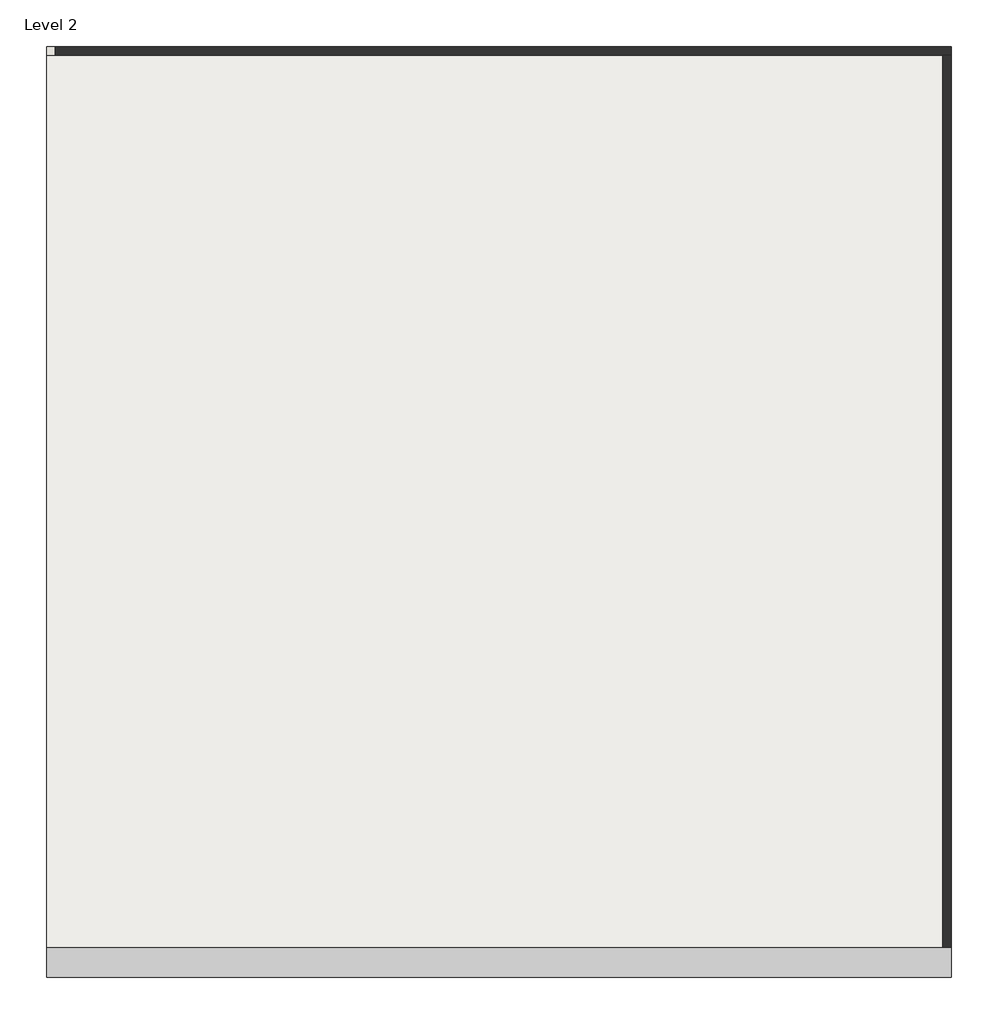
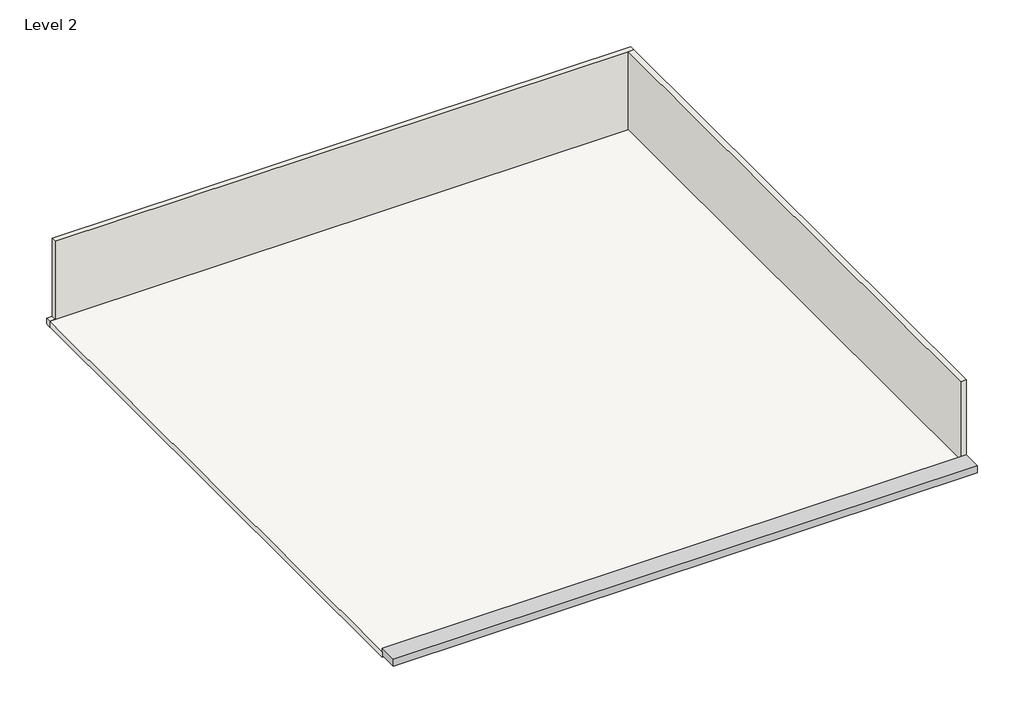
# One storey: 2 walls, 1 proxy, 1 roof.
"""IFC4 building model written with IfcOpenShell, lengths in millimetres."""

from ifc_helpers import new_model, si_unit, frame, origin, place, context, project, spatial, polyline, outline, extrude, faceted_brep, transform, mapped, element, save
from components import generic_models_1_generic_models_1_efd73d5e

model = new_model("IFC4")

# Units and contexts
model_context = context("Model", 3, world=origin())
ifc_project = project(units=[si_unit("LENGTHUNIT", "METRE", prefix="MILLI")], contexts=[model_context])

# Site, building, storey
site = spatial("IfcSite", under=ifc_project)
building = spatial("IfcBuilding", under=site)
storey = spatial("IfcBuildingStorey", under=building, Name="Level 2", Elevation=3048.0)

# Proxy
placement = place(None, origin())
generic_models_1_generic_models_1_shape = generic_models_1_generic_models_1_efd73d5e(model_context)
element("IfcBuildingElementProxy", 1, Name="Generic Models 1 : Generic Models 1", ObjectType="Generic Models 1 : Generic Models 1", at=placement, inside=storey, context=model_context, shape_type="MappedRepresentation", body=[
    mapped(generic_models_1_generic_models_1_shape, transform((0.0, 0.0, 0.0), x_axis=(1.0, 0.0, 0.0), y_axis=(0.0, 1.0, 0.0), z_axis=(0.0, 0.0, 1.0))),
])

# Roof
element("IfcRoof", 2, ObjectType="Generic - 9\"", at=placement, inside=storey, context=model_context, shape_type="SweptSolid", body=[
    extrude(outline(polyline([(-8934.7629849, 17755.0995758), (12604.4370151, 17755.0995758), (12604.4370151, -3682.5004242), (-8934.7629849, -3682.5004242), (-8934.7629849, 17755.0995758)])), frame((0.0, 0.0, 3048.0), z_axis=(0.0, 0.0, 1.0), x_axis=(1.0, 0.0, 0.0)), (0.0, 0.0, 1.0), 228.6),
])

# Walls
element("IfcWall", 3, ObjectType="outer wall", at=placement, inside=storey, context=model_context, shape_type="Brep", body=[
    faceted_brep([(-8934.7629849, 17551.8995758, 3048.0), (-8731.5629849, 17551.8995758, 3048.0), (12401.2370151, 17551.8995758, 3048.0), (12604.4370151, 17551.8995758, 3048.0), (12604.4370151, 17551.8995758, 6324.6), (12401.2370151, 17551.8995758, 6324.6), (-8731.5629849, 17551.8995758, 6324.6), (-8731.5629849, 17551.8995758, 3276.6), (-8934.7629849, 17551.8995758, 3276.6), (-8934.7629849, 17755.0995758, 3048.0), (-8934.7629849, 17755.0995758, 3276.6), (-8731.5629849, 17755.0995758, 3276.6), (-8731.5629849, 17755.0995758, 6324.6), (12604.4370151, 17755.0995758, 6324.6), (12604.4370151, 17755.0995758, 3048.0), (-8731.5629849, 17755.0995758, 3048.0)], [[[0, 1, 2, 3, 4, 5, 6, 7, 8]], [[9, 10, 11, 12, 13, 14, 15]], [[3, 2, 1, 0, 9, 15, 14]], [[6, 5, 4, 13, 12]], [[7, 11, 10, 8]], [[0, 8, 10, 9]], [[7, 6, 12, 11]], [[4, 3, 14, 13]]]),
])
element("IfcWall", 4, ObjectType="outer wall", at=placement, inside=storey, context=model_context, shape_type="SweptSolid", body=[
    extrude(outline(polyline([(12401.2370151, -3682.5004242), (12401.2370151, 17551.8995758), (12604.4370151, 17551.8995758), (12604.4370151, -3682.5004242), (12401.2370151, -3682.5004242)])), frame((0.0, 0.0, 3048.0), z_axis=(0.0, 0.0, 1.0), x_axis=(1.0, 0.0, 0.0)), (0.0, 0.0, 1.0), 3276.6),
])

save(model, "model.ifc")

# Revit data of these elements
# Type "Generic - 9\""
#   Assembly Code = "B1020"
#   Layers, outside or top first: 0' - 9" no material (function 1)
# Type "outer wall"
#   Assembly Code = "B2010"
#   Layers, outside or top first: 0' - 8" "Copper" (function 1)
# Element 1 (IfcBuildingElementProxy, "Generic Models 1 : Generic Models 1")
#   Phase Created = New Construction
# Element 2 (IfcRoof, "Generic - 9\"")
#   built-in parameter 1001705 = 10.75 (stored number, unit not read)
#   built-in parameter 1001710 = 33615
#   Phase Created = New Construction
#   Materials on its faces: "Default Roof"
# Elements 3, 4 (IfcWall, "outer wall")
#   Top Offset = 0' - 0"
#   Base Offset = 0' - 0"
#   Unconnected Height = 10' - 9"
#   wall height = 10' - 9"
#   Phase Created = New Construction
#   Base Constraint = Level 2
#   Materials on its faces: "Copper"
# Materials
#   "Copper": class "Metal", colour RGB 0 0 0, transparency 0, Description = "Copper, matte finish", Cost = 0
#   "Default Roof": colour RGB 88 101 114, transparency 0
